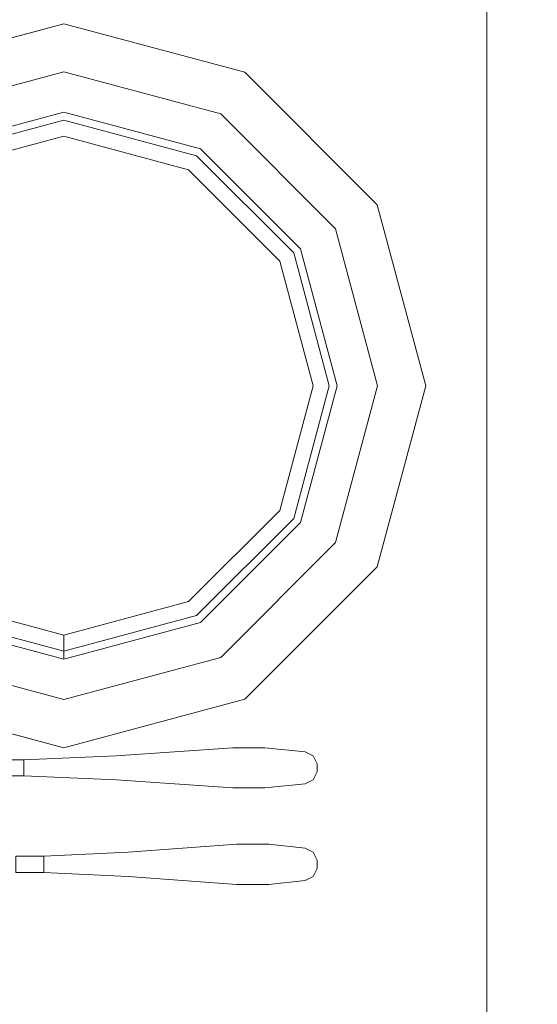
# Model space of a CAD drawing. Units: inches. Extents: x 375 to 1122, y 27 to 1069.
# Tile 113 of 155: x 739 to 747, y 860 to 875. Entities that reach past the tile are written whole.
import ezdxf

# ---------------------------------------------------------------- set-up
doc = ezdxf.new("R2010")
doc.units = ezdxf.units.IN
doc.layers.add('A-ANNO-DIMS', color=2, linetype='Continuous', lineweight=18)
doc.layers.add('Furniture', color=30, linetype='Continuous', lineweight=18)
doc.styles.get("Standard").update_dxf_attribs({"font": 'arial.ttf'})
doc.dimstyles.new('ISO-25', dxfattribs={"dimtxt": 12, "dimasz": 2.5, "dimexe": 1.5, "dimexo": 1.5, "dimtad": 1, "dimdec": 1, "dimlunit": 3, "dimtxsty": 'Standard', "dimblk": 'ARCHTICK', "dimcen": 2.5, "dimadec": 0, "dimazin": 0, "dimtfac": 1, "dimtdec": 1, "dimtmove": 0, "dimatfit": 3, "dimfxl": 1.5, "dimfxlon": 1, "dimarcsym": 0})

# ---------------------------------------------------------------- blocks, each defined once
blk = doc.blocks.new('A$C403C54AD')
blk.add_line((0.83575, 1.53256, -0.0006), (1.99923, 1.53256, -0.0006))
at = {"linetype": 'ByBlock'}
for points, invisible_edges in [([(1.72651, 1.50922, -0.02349), (1.72651, 1.49075, -0.02349), (1.66648, 1.47466, -0.02349), (1.65725, 1.49066, -0.02349)], 5), ([(1.72651, 1.47535, -0.03734), (1.72651, 1.50922, -0.02811), (1.65725, 1.49066, -0.02811), (1.67418, 1.46133, -0.03734)], 5), ([(1.79578, 1.49066, -0.02349), (1.78654, 1.47466, -0.02349), (1.72651, 1.49075, -0.02349), (1.72651, 1.50922, -0.02349)], 5), ([(1.77884, 1.46133, -0.03734), (1.79578, 1.49066, -0.02811), (1.72651, 1.50922, -0.02811), (1.72651, 1.47535, -0.03734)], 5), ([(1.65725, 1.49066, -0.02349), (1.66648, 1.47466, -0.02349), (1.62254, 1.43072, -0.02349), (1.60654, 1.43995, -0.02349)], 5), ([(1.67418, 1.46133, -0.03734), (1.65725, 1.49066, -0.02811), (1.60654, 1.43995, -0.02811), (1.63587, 1.42302, -0.03734)], 5), ([(1.72651, 1.49075, -0.02349), (1.72651, 1.47228, -0.02965), (1.67572, 1.45867, -0.02965), (1.66648, 1.47466, -0.02349)], 5), ([(1.78654, 1.47466, -0.02349), (1.7773, 1.45867, -0.02965), (1.72651, 1.47228, -0.02965), (1.72651, 1.49075, -0.02349)], 5), ([(1.81715, 1.42302, -0.03734), (1.84648, 1.43995, -0.02811), (1.79578, 1.49066, -0.02811), (1.77884, 1.46133, -0.03734)], 5), ([(1.84648, 1.43995, -0.02349), (1.83048, 1.43072, -0.02349), (1.78654, 1.47466, -0.02349), (1.79578, 1.49066, -0.02349)], 5), ([(1.66648, 1.47466, -0.02349), (1.67572, 1.45867, -0.02965), (1.63853, 1.42148, -0.02965), (1.62254, 1.43072, -0.02349)], 5), ([(1.72651, 1.46612, -0.04658), (1.72651, 1.47535, -0.03734), (1.67418, 1.46133, -0.03734), (1.6788, 1.45333, -0.04658)], 5), ([(1.77423, 1.45333, -0.04658), (1.77884, 1.46133, -0.03734), (1.72651, 1.47535, -0.03734), (1.72651, 1.46612, -0.04658)], 5), ([(1.83048, 1.43072, -0.02349), (1.81449, 1.42148, -0.02965), (1.7773, 1.45867, -0.02965), (1.78654, 1.47466, -0.02349)], 5), ([(1.72651, 1.47228, -0.02965), (1.72651, 1.37069, -0.02965), (1.72651, 1.37069, -0.02965), (1.67572, 1.45867, -0.02965)], 5), ([(1.7773, 1.45867, -0.02965), (1.72651, 1.37069, -0.02965), (1.72651, 1.37069, -0.02965), (1.72651, 1.47228, -0.02965)], 5), ([(1.6788, 1.45333, -0.04658), (1.67418, 1.46133, -0.03734), (1.63587, 1.42302, -0.03734), (1.64387, 1.4184, -0.04658)], 5), ([(1.67572, 1.45867, -0.02965), (1.72651, 1.37069, -0.02965), (1.72651, 1.37069, -0.02965), (1.63853, 1.42148, -0.02965)], 5), ([(1.81449, 1.42148, -0.02965), (1.72651, 1.37069, -0.02965), (1.72651, 1.37069, -0.02965), (1.7773, 1.45867, -0.02965)], 5), ([(1.80916, 1.4184, -0.04658), (1.81715, 1.42302, -0.03734), (1.77884, 1.46133, -0.03734), (1.77423, 1.45333, -0.04658)], 5), ([(1.60654, 1.43995, -0.02349), (1.62254, 1.43072, -0.02349), (1.60645, 1.37069, -0.02349), (1.58798, 1.37069, -0.02349)], 5), ([(1.63587, 1.42302, -0.03734), (1.60654, 1.43995, -0.02811), (1.58798, 1.37069, -0.02811), (1.62185, 1.37069, -0.03734)], 5), ([(1.83118, 1.37069, -0.03734), (1.86504, 1.37069, -0.02811), (1.84648, 1.43995, -0.02811), (1.81715, 1.42302, -0.03734)], 5), ([(1.86504, 1.37069, -0.02349), (1.84657, 1.37069, -0.02349), (1.83048, 1.43072, -0.02349), (1.84648, 1.43995, -0.02349)], 5), ([(1.62254, 1.43072, -0.02349), (1.63853, 1.42148, -0.02965), (1.62492, 1.37069, -0.02965), (1.60645, 1.37069, -0.02349)], 5), ([(1.84657, 1.37069, -0.02349), (1.8281, 1.37069, -0.02965), (1.81449, 1.42148, -0.02965), (1.83048, 1.43072, -0.02349)], 5), ([(1.64387, 1.4184, -0.04658), (1.63587, 1.42302, -0.03734), (1.62185, 1.37069, -0.03734), (1.63108, 1.37069, -0.04658)], 5), ([(1.63853, 1.42148, -0.02965), (1.72651, 1.37069, -0.02965), (1.72651, 1.37069, -0.02965), (1.62492, 1.37069, -0.02965)], 5), ([(1.8281, 1.37069, -0.02965), (1.72651, 1.37069, -0.02965), (1.72651, 1.37069, -0.02965), (1.81449, 1.42148, -0.02965)], 5), ([(1.82194, 1.37069, -0.04658), (1.83118, 1.37069, -0.03734), (1.81715, 1.42302, -0.03734), (1.80916, 1.4184, -0.04658)], 4), ([(1.58798, 1.37069, -0.02349), (1.60645, 1.37069, -0.02349), (1.62254, 1.31066, -0.02349), (1.60654, 1.30143, -0.02349)], 5), ([(1.62185, 1.37069, -0.03734), (1.58798, 1.37069, -0.02811), (1.60654, 1.30143, -0.02811), (1.63587, 1.31836, -0.03734)], 5), ([(1.60645, 1.37069, -0.02349), (1.62492, 1.37069, -0.02965), (1.63853, 1.3199, -0.02965), (1.62254, 1.31066, -0.02349)], 5), ([(1.63108, 1.37069, -0.04658), (1.62185, 1.37069, -0.03734), (1.63587, 1.31836, -0.03734), (1.64387, 1.32297, -0.04658)], 5), ([(1.62492, 1.37069, -0.02965), (1.72651, 1.37069, -0.02965), (1.72651, 1.37069, -0.02965), (1.63853, 1.3199, -0.02965)], 5), ([(1.63853, 1.3199, -0.02965), (1.72651, 1.37069, -0.02965), (1.72651, 1.37069, -0.02965), (1.67572, 1.28271, -0.02965)], 5), ([(1.67572, 1.28271, -0.02965), (1.72651, 1.37069, -0.02965), (1.72651, 1.37069, -0.02965), (1.72651, 1.2691, -0.02965)], 5), ([(1.72651, 1.2691, -0.02965), (1.72651, 1.37069, -0.02965), (1.72651, 1.37069, -0.02965), (1.7773, 1.28271, -0.02965)], 5), ([(1.81449, 1.3199, -0.02965), (1.72651, 1.37069, -0.02965), (1.72651, 1.37069, -0.02965), (1.8281, 1.37069, -0.02965)], 5), ([(1.7773, 1.28271, -0.02965), (1.72651, 1.37069, -0.02965), (1.72651, 1.37069, -0.02965), (1.81449, 1.3199, -0.02965)], 5), ([(1.83048, 1.31066, -0.02349), (1.81449, 1.3199, -0.02965), (1.8281, 1.37069, -0.02965), (1.84657, 1.37069, -0.02349)], 5), ([(1.81715, 1.31836, -0.03734), (1.84648, 1.30143, -0.02811), (1.86504, 1.37069, -0.02811), (1.83118, 1.37069, -0.03734)], 5), ([(1.84648, 1.30143, -0.02349), (1.83048, 1.31066, -0.02349), (1.84657, 1.37069, -0.02349), (1.86504, 1.37069, -0.02349)], 5)]:
    blk.add_3dface(points, dxfattribs=dict(at, invisible_edges=invisible_edges))
for points in [[(1.72651, 1.50922, -0.02811), (1.72651, 1.50922, -0.02349), (1.65725, 1.49066, -0.02349), (1.65725, 1.49066, -0.02811)], [(1.79578, 1.49066, -0.02811), (1.79578, 1.49066, -0.02349), (1.72651, 1.50922, -0.02349), (1.72651, 1.50922, -0.02811)], [(1.65725, 1.49066, -0.02811), (1.65725, 1.49066, -0.02349), (1.60654, 1.43995, -0.02349), (1.60654, 1.43995, -0.02811)], [(1.84648, 1.43995, -0.02811), (1.84648, 1.43995, -0.02349), (1.79578, 1.49066, -0.02349), (1.79578, 1.49066, -0.02811)], [(1.60654, 1.43995, -0.02811), (1.60654, 1.43995, -0.02349), (1.58798, 1.37069, -0.02349), (1.58798, 1.37069, -0.02811)], [(1.86504, 1.37069, -0.02811), (1.86504, 1.37069, -0.02349), (1.84648, 1.43995, -0.02349), (1.84648, 1.43995, -0.02811)], [(1.58798, 1.37069, -0.02811), (1.58798, 1.37069, -0.02349), (1.60654, 1.30143, -0.02349), (1.60654, 1.30143, -0.02811)], [(1.80916, 1.32297, -0.04658), (1.81715, 1.31836, -0.03734), (1.83118, 1.37069, -0.03734), (1.82194, 1.37069, -0.04658)], [(1.84648, 1.30143, -0.02811), (1.84648, 1.30143, -0.02349), (1.86504, 1.37069, -0.02349), (1.86504, 1.37069, -0.02811)]]:
    blk.add_3dface(points, dxfattribs=at)
for points, invisible_edges in [([(1.86812, 1.46612, -0.03397), (1.87735, 1.46612, -0.03397), (1.87889, 1.46304, -0.03421), (1.86658, 1.46304, -0.03421)], 5), ([(1.86812, 1.46612, -0.0386), (1.87735, 1.46612, -0.0386), (1.87889, 1.46304, -0.03884), (1.86658, 1.46304, -0.03884)], 5), ([(1.87427, 1.46766, -0.03413), (1.8712, 1.46766, -0.03413), (1.86812, 1.46612, -0.03397), (1.87735, 1.46612, -0.03397)], 4), ([(1.87427, 1.46766, -0.03827), (1.8712, 1.46766, -0.03827), (1.86812, 1.46612, -0.0386), (1.87735, 1.46612, -0.0386)], 4), ([(1.90506, 1.46612, -0.03397), (1.91429, 1.46612, -0.03397), (1.91583, 1.46304, -0.03421), (1.90352, 1.46304, -0.03421)], 5), ([(1.90506, 1.46612, -0.0386), (1.91429, 1.46612, -0.0386), (1.91583, 1.46304, -0.03884), (1.90352, 1.46304, -0.03884)], 5), ([(1.91121, 1.46766, -0.03413), (1.90814, 1.46766, -0.03413), (1.90506, 1.46612, -0.03397), (1.91429, 1.46612, -0.03397)], 4), ([(1.91121, 1.46766, -0.03827), (1.90814, 1.46766, -0.03827), (1.90506, 1.46612, -0.0386), (1.91429, 1.46612, -0.0386)], 4), ([(1.87889, 1.46304, -0.03421), (1.86658, 1.46304, -0.03421), (1.86504, 1.44765, -0.03425), (1.88043, 1.44765, -0.03425)], 5), ([(1.87889, 1.46304, -0.03884), (1.86658, 1.46304, -0.03884), (1.86504, 1.44765, -0.03888), (1.88043, 1.44765, -0.03888)], 5), ([(1.91583, 1.46304, -0.03421), (1.90352, 1.46304, -0.03421), (1.90198, 1.44919, -0.03425), (1.91737, 1.44919, -0.03425)], 5), ([(1.91583, 1.46304, -0.03884), (1.90352, 1.46304, -0.03884), (1.90198, 1.44919, -0.03888), (1.91737, 1.44919, -0.03888)], 5), ([(1.86504, 1.44765, -0.03425), (1.88043, 1.44765, -0.03425), (1.88043, 1.43534, -0.03392), (1.86504, 1.43534, -0.03392)], 5), ([(1.86504, 1.44765, -0.03888), (1.88043, 1.44765, -0.03888), (1.88043, 1.43534, -0.03855), (1.86504, 1.43534, -0.03855)], 5), ([(1.90198, 1.44919, -0.03425), (1.91737, 1.44919, -0.03425), (1.91737, 1.43687, -0.03392), (1.90198, 1.43687, -0.03392)], 5), ([(1.90198, 1.44919, -0.03888), (1.91737, 1.44919, -0.03888), (1.91737, 1.43687, -0.03855), (1.90198, 1.43687, -0.03855)], 5), ([(1.91737, 1.43687, -0.03392), (1.90198, 1.43687, -0.03392), (1.90506, 1.39532, -0.03153), (1.91429, 1.39532, -0.03153)], 5), ([(1.91737, 1.43687, -0.03855), (1.90198, 1.43687, -0.03855), (1.90506, 1.39532, -0.03461), (1.91429, 1.39532, -0.03461)], 5), ([(1.90198, 1.43687, -0.03855), (1.90198, 1.43687, -0.03392), (1.90506, 1.39532, -0.03153), (1.90506, 1.39532, -0.03461)], 4), ([(1.91429, 1.39532, -0.03461), (1.91429, 1.39532, -0.03153), (1.91737, 1.43687, -0.03392), (1.91737, 1.43687, -0.03855)], 1), ([(1.88043, 1.43534, -0.03392), (1.86504, 1.43534, -0.03392), (1.86812, 1.3907, -0.03153), (1.87735, 1.3907, -0.03153)], 5), ([(1.88043, 1.43534, -0.03855), (1.86504, 1.43534, -0.03855), (1.86812, 1.3907, -0.03461), (1.87735, 1.3907, -0.03461)], 5), ([(1.86504, 1.43534, -0.03855), (1.86504, 1.43534, -0.03392), (1.86812, 1.3907, -0.03153), (1.86812, 1.3907, -0.03461)], 4), ([(1.87735, 1.3907, -0.03461), (1.87735, 1.3907, -0.03153), (1.88043, 1.43534, -0.03392), (1.88043, 1.43534, -0.03855)], 1), ([(1.90506, 1.39532, -0.03153), (1.91429, 1.39532, -0.03153), (1.91275, 1.36299, -0.02863), (1.9066, 1.36299, -0.02863)], 1), ([(1.90506, 1.39532, -0.03153), (1.90506, 1.39532, -0.03461), (1.9066, 1.36299, -0.03122), (1.9066, 1.36299, -0.02863)], 5), ([(1.90506, 1.39532, -0.03461), (1.91429, 1.39532, -0.03461), (1.91275, 1.36299, -0.03122), (1.9066, 1.36299, -0.03122)], 1), ([(1.91275, 1.36299, -0.02863), (1.91275, 1.36299, -0.03122), (1.91429, 1.39532, -0.03461), (1.91429, 1.39532, -0.03153)], 5), ([(1.86812, 1.3907, -0.03153), (1.87735, 1.3907, -0.03153), (1.87581, 1.3553, -0.02863), (1.86966, 1.3553, -0.02863)], 1), ([(1.86812, 1.3907, -0.03153), (1.86812, 1.3907, -0.03461), (1.86966, 1.3553, -0.03122), (1.86966, 1.3553, -0.02863)], 5), ([(1.86812, 1.3907, -0.03461), (1.87735, 1.3907, -0.03461), (1.87581, 1.3553, -0.03122), (1.86966, 1.3553, -0.03122)], 1), ([(1.87581, 1.3553, -0.02863), (1.87581, 1.3553, -0.03122), (1.87735, 1.3907, -0.03461), (1.87735, 1.3907, -0.03153)], 5), ([(1.9066, 1.36299, -0.03122), (1.9066, 1.36299, -0.02863), (1.9066, 1.35222, -0.03071), (1.9066, 1.35222, -0.0333)], 5), ([(1.91275, 1.35222, -0.0333), (1.91275, 1.35222, -0.03071), (1.91275, 1.36299, -0.02863), (1.91275, 1.36299, -0.03122)], 5), ([(1.86966, 1.3553, -0.03122), (1.86966, 1.3553, -0.02863), (1.86966, 1.34452, -0.03071), (1.86966, 1.34452, -0.0333)], 5), ([(1.87581, 1.34452, -0.0333), (1.87581, 1.34452, -0.03071), (1.87581, 1.3553, -0.02863), (1.87581, 1.3553, -0.03122)], 5)]:
    blk.add_3dface(points, dxfattribs=dict(invisible_edges=invisible_edges))
for points in [[(1.86812, 1.46612, -0.03397), (1.86812, 1.46612, -0.0386), (1.86658, 1.46304, -0.03884), (1.86658, 1.46304, -0.03421)], [(1.8712, 1.46766, -0.03827), (1.8712, 1.46766, -0.03413), (1.86812, 1.46612, -0.03397), (1.86812, 1.46612, -0.0386)], [(1.87427, 1.46766, -0.03413), (1.87427, 1.46766, -0.03827), (1.8712, 1.46766, -0.03827), (1.8712, 1.46766, -0.03413)], [(1.87735, 1.46612, -0.0386), (1.87735, 1.46612, -0.03397), (1.87427, 1.46766, -0.03413), (1.87427, 1.46766, -0.03827)], [(1.87889, 1.46304, -0.03421), (1.87889, 1.46304, -0.03884), (1.87735, 1.46612, -0.0386), (1.87735, 1.46612, -0.03397)], [(1.90506, 1.46612, -0.03397), (1.90506, 1.46612, -0.0386), (1.90352, 1.46304, -0.03884), (1.90352, 1.46304, -0.03421)], [(1.90814, 1.46766, -0.03827), (1.90814, 1.46766, -0.03413), (1.90506, 1.46612, -0.03397), (1.90506, 1.46612, -0.0386)], [(1.91121, 1.46766, -0.03413), (1.91121, 1.46766, -0.03827), (1.90814, 1.46766, -0.03827), (1.90814, 1.46766, -0.03413)], [(1.91429, 1.46612, -0.0386), (1.91429, 1.46612, -0.03397), (1.91121, 1.46766, -0.03413), (1.91121, 1.46766, -0.03827)], [(1.91583, 1.46304, -0.03421), (1.91583, 1.46304, -0.03884), (1.91429, 1.46612, -0.0386), (1.91429, 1.46612, -0.03397)], [(1.86658, 1.46304, -0.03884), (1.86658, 1.46304, -0.03421), (1.86504, 1.44765, -0.03425), (1.86504, 1.44765, -0.03888)], [(1.88043, 1.44765, -0.03888), (1.88043, 1.44765, -0.03425), (1.87889, 1.46304, -0.03421), (1.87889, 1.46304, -0.03884)], [(1.90352, 1.46304, -0.03884), (1.90352, 1.46304, -0.03421), (1.90198, 1.44919, -0.03425), (1.90198, 1.44919, -0.03888)], [(1.91737, 1.44919, -0.03888), (1.91737, 1.44919, -0.03425), (1.91583, 1.46304, -0.03421), (1.91583, 1.46304, -0.03884)], [(1.86504, 1.44765, -0.03425), (1.86504, 1.44765, -0.03888), (1.86504, 1.43534, -0.03855), (1.86504, 1.43534, -0.03392)], [(1.88043, 1.43534, -0.03392), (1.88043, 1.43534, -0.03855), (1.88043, 1.44765, -0.03888), (1.88043, 1.44765, -0.03425)], [(1.90198, 1.44919, -0.03425), (1.90198, 1.44919, -0.03888), (1.90198, 1.43687, -0.03855), (1.90198, 1.43687, -0.03392)], [(1.91737, 1.43687, -0.03392), (1.91737, 1.43687, -0.03855), (1.91737, 1.44919, -0.03888), (1.91737, 1.44919, -0.03425)], [(1.91275, 1.36299, -0.02863), (1.9066, 1.36299, -0.02863), (1.9066, 1.35222, -0.03071), (1.91275, 1.35222, -0.03071)], [(1.91275, 1.36299, -0.03122), (1.9066, 1.36299, -0.03122), (1.9066, 1.35222, -0.0333), (1.91275, 1.35222, -0.0333)], [(1.87581, 1.3553, -0.02863), (1.86966, 1.3553, -0.02863), (1.86966, 1.34452, -0.03071), (1.87581, 1.34452, -0.03071)], [(1.87581, 1.3553, -0.03122), (1.86966, 1.3553, -0.03122), (1.86966, 1.34452, -0.0333), (1.87581, 1.34452, -0.0333)]]:
    blk.add_3dface(points)
blk = doc.blocks.new('_ArchTick')
at = {"color": 0, "linetype": 'ByBlock', "const_width": 0.15}
blk.add_lwpolyline([(-0.5, -0.5), (0.5, 0.5)], dxfattribs=at)
blk = doc.blocks.new('*D85')
at = {"layer": 'A-ANNO-DIMS', "color": 0, "lineweight": -2, "transparency": 16777216}
for p, q in [((401.507, 868.528), (398.507, 868.528)), ((400.007, 814.528), (400.007, 868.528)), ((401.507, 814.528), (398.507, 814.528))]:
    blk.add_line(p, q, dxfattribs=at)
at = {"layer": 'Defpoints', "color": 0, "transparency": 16777216}
for p in [(400.007, 868.528), (845.007, 868.528), (845.007, 814.528)]:
    blk.add_point(p, dxfattribs=at)
at = {"layer": 'A-ANNO-DIMS', "color": 0, "lineweight": -2, "transparency": 16777216, "xscale": 2.5, "yscale": 2.5, "zscale": 2.5}
for p, rotation in [((400.007, 868.528), 90), ((400.007, 814.528), 270)]:
    blk.add_blockref('_ArchTick', p, dxfattribs=dict(at, rotation=rotation))
at = {"layer": 'A-ANNO-DIMS', "color": 0, "transparency": 16777216, "insert": (393.255, 841.528), "char_height": 12, "attachment_point": 5, "rotation": 90}
blk.add_mtext('4\'-6"', dxfattribs=at)
blk = doc.blocks.new('*D88')
at = {"layer": 'A-ANNO-DIMS', "color": 0, "lineweight": -2, "transparency": 16777216}
for p, q in [((731.007, 1052.528), (731.007, 1055.528)), ((854.007, 1052.528), (854.007, 1055.528)), ((731.007, 1054.028), (854.007, 1054.028))]:
    blk.add_line(p, q, dxfattribs=at)
at = {"layer": 'Defpoints', "color": 0, "transparency": 16777216}
for p in [(854.007, 1054.028), (731.007, 502.528), (854.007, 502.528)]:
    blk.add_point(p, dxfattribs=at)
at = {"layer": 'A-ANNO-DIMS', "color": 0, "lineweight": -2, "transparency": 16777216, "xscale": 2.5, "yscale": 2.5, "zscale": 2.5, "rotation": 180}
blk.add_blockref('_ArchTick', (731.007, 1054.028), dxfattribs=at)
at = {"layer": 'A-ANNO-DIMS', "color": 0, "lineweight": -2, "transparency": 16777216, "xscale": 2.5, "yscale": 2.5, "zscale": 2.5}
blk.add_blockref('_ArchTick', (854.007, 1054.028), dxfattribs=at)
at = {"layer": 'A-ANNO-DIMS', "color": 0, "transparency": 16777216, "insert": (792.507, 1060.784), "char_height": 12, "attachment_point": 5}
blk.add_mtext('10\'-3"', dxfattribs=at)
blk = doc.blocks.new('*D91')
at = {"layer": 'A-ANNO-DIMS', "color": 0, "lineweight": -2, "transparency": 16777216}
for p, q in [((728.007, 1052.528), (728.007, 1055.528)), ((788.007, 1052.528), (788.007, 1055.528)), ((728.007, 1054.028), (788.007, 1054.028))]:
    blk.add_line(p, q, dxfattribs=at)
at = {"layer": 'Defpoints', "color": 0, "transparency": 16777216}
for p in [(788.007, 1054.028), (728.007, 774.028), (788.007, 774.028)]:
    blk.add_point(p, dxfattribs=at)
at = {"layer": 'A-ANNO-DIMS', "color": 0, "lineweight": -2, "transparency": 16777216, "xscale": 2.5, "yscale": 2.5, "zscale": 2.5, "rotation": 180}
blk.add_blockref('_ArchTick', (728.007, 1054.028), dxfattribs=at)
at = {"layer": 'A-ANNO-DIMS', "color": 0, "lineweight": -2, "transparency": 16777216, "xscale": 2.5, "yscale": 2.5, "zscale": 2.5}
blk.add_blockref('_ArchTick', (788.007, 1054.028), dxfattribs=at)
at = {"layer": 'A-ANNO-DIMS', "color": 0, "transparency": 16777216, "insert": (758.007, 1060.78), "char_height": 12, "attachment_point": 5}
blk.add_mtext('5\'-0"', dxfattribs=at)

msp = doc.modelspace()

# ---------------------------------------------------------------- block references
at = {"layer": 'Furniture', "xscale": 39.9918517141215, "yscale": 39.9918517141215, "zscale": 39.9918517141215, "rotation": 270}
msp.add_blockref('A$C403C54AD', (684.955, 938.316, 0.024), dxfattribs=at)

# ---------------------------------------------------------------- dimensions: what is measured, and where the dimension line sits
at = {"layer": 'A-ANNO-DIMS'}
for base, p1, p2, picture, middle in [((788.007, 1054.028), (728.007, 774.028), (788.007, 774.028), '*D91', (758.007, 1060.78)), ((854.007, 1054.028), (731.007, 502.528), (854.007, 502.528), '*D88', (792.507, 1060.784))]:
    dim = msp.add_linear_dim(base=base, p1=p1, p2=p2, dimstyle='ISO-25', override={"dimdec": 1, "dimlfac": 1, "dimrnd": 0, "dimzin": 1, "dimdsep": 46, "dimlunit": 4, "dimfrac": 2}, dxfattribs=at)
    dim.commit()
    dim.dimension.update_dxf_attribs({"geometry": picture, "text_midpoint": middle})
dim = msp.add_linear_dim(base=(400.007, 868.528), p1=(845.007, 814.528), p2=(845.007, 868.528), angle=90, dimstyle='ISO-25', override={"dimdec": 1, "dimlfac": 1, "dimrnd": 0, "dimzin": 1, "dimdsep": 46, "dimlunit": 4, "dimfrac": 2}, dxfattribs=at)
dim.commit()
dim.dimension.update_dxf_attribs({"geometry": '*D85', "text_midpoint": (393.255, 841.528)})

doc.saveas('drawing.dxf')
